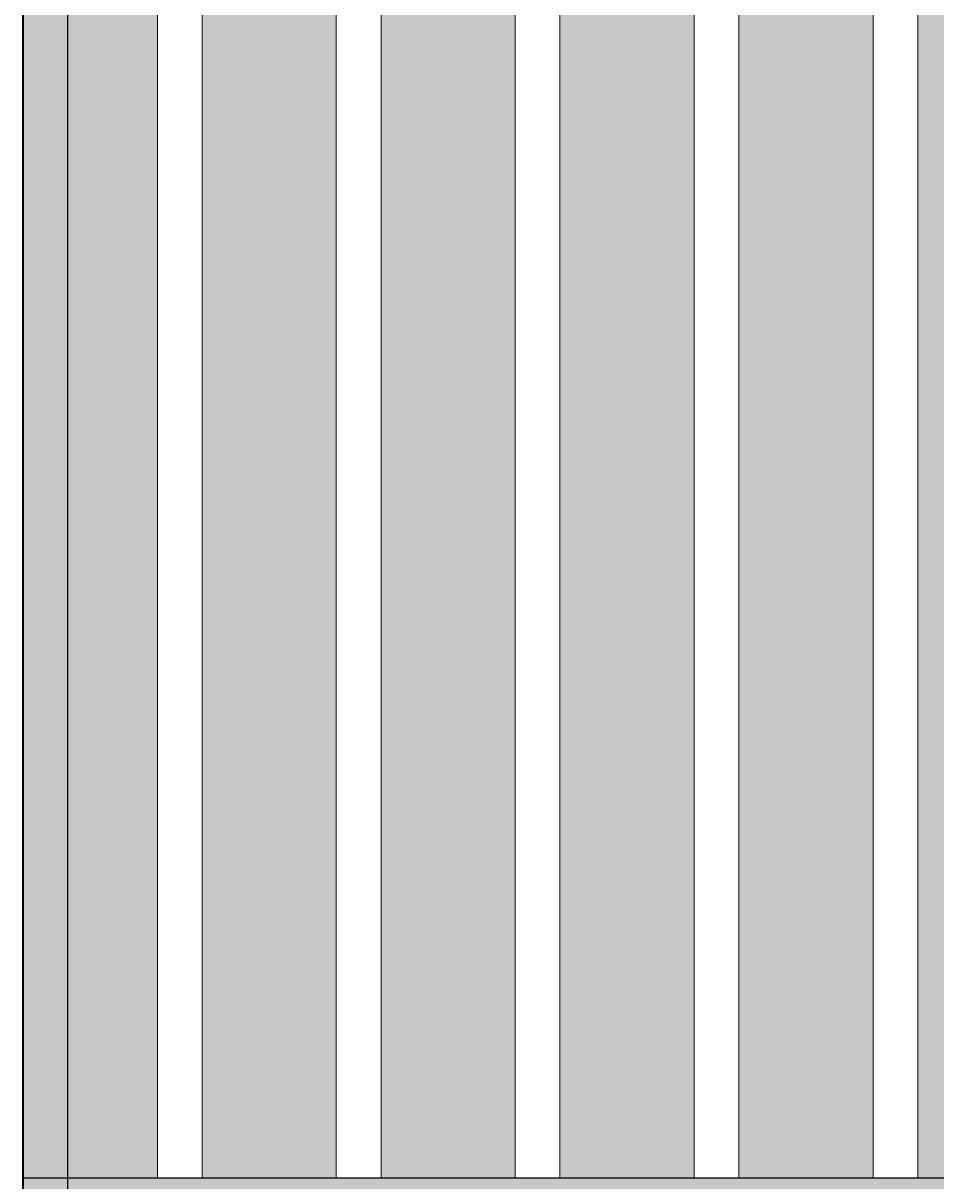
# Model space of a CAD drawing. Units: inches. Extents: x 4508 to 4723, y 847 to 1020.
# Tile 9 of 32: x 4550 to 4570, y 905 to 931. Entities that reach past the tile are written whole.
import ezdxf

# ---------------------------------------------------------------- set-up
doc = ezdxf.new("R2010")
doc.units = ezdxf.units.IN
for name, color, linetype, lineweight in [('A-ANNO-DIMS', 2, 'Continuous', 18), ('A-FURN', 8, 'Continuous', 25), ('A-WALL', 7, 'Continuous', 35), ('A-WALL-FINS', 30, 'Continuous', 18), ('A-WALL-PATT', 254, 'Continuous', 13)]:
    doc.layers.add(name, color=color, linetype=linetype, lineweight=lineweight)
doc.styles.get("Standard").update_dxf_attribs({"font": 'arial.ttf'})
doc.dimstyles.get("Standard").update_dxf_attribs({"dimtxt": 0.18, "dimasz": 0.18, "dimexe": 0.18, "dimexo": 0.0625, "dimgap": 0.09, "dimtad": 0, "dimtih": 1, "dimtoh": 1, "dimdec": 4, "dimzin": 0, "dimdsep": 46, "dimtxsty": 'Standard', "dimcen": 0.09, "dimadec": 0, "dimazin": 0, "dimtfac": 1, "dimtdec": 4, "dimtofl": 0, "dimtmove": 0, "dimatfit": 3, "dimfxl": 1, "dimtolj": 1, "dimtzin": 0, "dimarcsym": 0})

# ---------------------------------------------------------------- blocks, each defined once
blk = doc.blocks.new('*D26')
at = {"layer": 'A-ANNO-DIMS', "color": 0, "lineweight": -2, "transparency": 16777216}
for p, q in [((4549.994, 904.809), (4549.994, 1002.877)), ((4550.994, 903.809), (4550.994, 1002.877)), ((4550.174, 1002.697), (4550.371, 1002.697)), ((4550.814, 1002.697), (4550.617, 1002.697))]:
    blk.add_line(p, q, dxfattribs=at)
at = {"layer": 'A-ANNO-DIMS', "color": 0, "lineweight": 9, "transparency": 16777216}
for points in [[(4550.174, 1002.727), (4550.174, 1002.667), (4549.994, 1002.697)], [(4550.814, 1002.727), (4550.814, 1002.667), (4550.994, 1002.697)]]:
    blk.add_solid(points, dxfattribs=at)
at = {"layer": 'Defpoints', "color": 0, "lineweight": 9, "transparency": 16777216}
for p in [(4550.994, 1002.697), (4549.994, 904.747), (4550.994, 903.747)]:
    blk.add_point(p, dxfattribs=at)
at = {"layer": 'A-ANNO-DIMS', "color": 0, "transparency": 16777216, "insert": (4550.494, 1002.697), "char_height": 0.18, "attachment_point": 5}
blk.add_mtext('\\A1;1', dxfattribs=at)
blk = doc.blocks.new('*D27')
at = {"layer": 'A-ANNO-DIMS', "color": 0, "lineweight": -2, "transparency": 16777216}
for p, q in [((4550.994, 903.809), (4550.994, 1002.877)), ((4577.494, 903.809), (4577.494, 1002.877)), ((4551.174, 1002.697), (4563.918, 1002.697)), ((4577.314, 1002.697), (4564.57, 1002.697))]:
    blk.add_line(p, q, dxfattribs=at)
at = {"layer": 'A-ANNO-DIMS', "color": 0, "lineweight": 9, "transparency": 16777216}
for points in [[(4551.174, 1002.727), (4551.174, 1002.667), (4550.994, 1002.697)], [(4577.314, 1002.727), (4577.314, 1002.667), (4577.494, 1002.697)]]:
    blk.add_solid(points, dxfattribs=at)
at = {"layer": 'Defpoints', "color": 0, "lineweight": 9, "transparency": 16777216}
for p in [(4577.494, 1002.697), (4550.994, 903.747), (4577.494, 903.747)]:
    blk.add_point(p, dxfattribs=at)
at = {"layer": 'A-ANNO-DIMS', "color": 0, "transparency": 16777216, "insert": (4564.244, 1002.697), "char_height": 0.18, "attachment_point": 5}
blk.add_mtext('\\A1;26.5', dxfattribs=at)

msp = doc.modelspace()

# ---------------------------------------------------------------- hatches: boundary and pattern name
at = {"layer": 'A-WALL-PATT', "transparency": 33554681}
h = msp.add_hatch(color=256, dxfattribs=at)
h.dxf.hatch_style = 1
h.paths.add_polyline_path([(4552.9938, 994.7469), (4549.9938, 994.7469), (4549.9938, 904.7469), (4552.9938, 904.7469)])
h.paths.add_polyline_path([(4556.9938, 994.7469), (4553.9938, 994.7469), (4553.9938, 904.7469), (4556.9938, 904.7469)])
h.paths.add_polyline_path([(4560.9938, 994.7469), (4557.9938, 994.7469), (4557.9938, 904.7469), (4560.9938, 904.7469)])
h.paths.add_polyline_path([(4564.9938, 994.7469), (4561.9938, 994.7469), (4561.9938, 904.7469), (4564.9938, 904.7469)])
h.paths.add_polyline_path([(4568.9938, 994.7469), (4565.9938, 994.7469), (4565.9938, 904.7469), (4568.9938, 904.7469)])
h.paths.add_polyline_path([(4572.9938, 994.7469), (4569.9938, 994.7469), (4569.9938, 904.7469), (4572.9938, 904.7469)])
h.paths.add_polyline_path([(4576.9938, 994.7469), (4573.9938, 994.7469), (4573.9938, 904.7469), (4576.9938, 904.7469)])
h.paths.add_polyline_path([(4580.9938, 994.7469), (4577.9938, 994.7469), (4577.9938, 904.7469), (4580.9938, 904.7469)])
h.paths.add_polyline_path([(4584.9938, 994.7469), (4581.9938, 994.7469), (4581.9938, 904.7469), (4584.9938, 904.7469)])
h = msp.add_hatch(color=256, dxfattribs=at)
h.dxf.hatch_style = 1
h.paths.add_polyline_path([(4577.4938, 903.7469), (4550.9938, 903.7469), (4550.9938, 887.7469), (4577.4938, 887.7469)], flags=0)
h.paths.add_polyline_path([(4603.9938, 903.7469), (4577.9938, 903.7469), (4577.9938, 887.7469), (4603.9938, 887.7469)], flags=0)
h.paths.add_polyline_path([(4656.9938, 903.7469), (4630.9938, 903.7469), (4630.9938, 887.7469), (4656.9938, 887.7469)], flags=0)
h.paths.add_polyline_path([(4657.9938, 904.7469), (4549.9938, 904.7469), (4549.9938, 886.7469), (4657.9938, 886.7469)])
h.paths.add_polyline_path([(4656.9938, 903.7469), (4656.9938, 887.7469), (4550.9938, 887.7469), (4550.9938, 903.7469)], flags=16)

# ---------------------------------------------------------------- linework, layer by layer
at = {"layer": 'A-FURN'}
msp.add_lwpolyline([(4657.9938, 886.7469), (4549.9938, 886.7469), (4549.9938, 904.7469), (4657.9938, 904.7469)], close=True, dxfattribs=at)
at = {"layer": 'A-WALL'}
msp.add_line((4549.9938, 874.7469), (4549.9938, 994.7469), dxfattribs=at)
at = {"layer": 'A-WALL-FINS'}
for p, q in [((4552.9938, 904.7469), (4552.9938, 994.7469)), ((4553.9938, 904.7469), (4553.9938, 994.7469)), ((4556.9938, 904.7469), (4556.9938, 994.7469)), ((4557.9938, 904.7469), (4557.9938, 994.7469)), ((4560.9938, 904.7469), (4560.9938, 994.7469)), ((4561.9938, 904.7469), (4561.9938, 994.7469)), ((4564.9938, 904.7469), (4564.9938, 994.7469)), ((4565.9938, 904.7469), (4565.9938, 994.7469)), ((4568.9938, 904.7469), (4568.9938, 994.7469)), ((4569.9938, 904.7469), (4569.9938, 994.7469))]:
    msp.add_line(p, q, dxfattribs=at)

# ---------------------------------------------------------------- dimensions: what is measured, and where the dimension line sits
at = {"layer": 'A-ANNO-DIMS'}
for base, p1, p2, override, picture, middle in [((4550.9938, 1002.6969), (4549.9938, 904.7469), (4550.9938, 903.7469), {"dimdec": 0, "dimlfac": 1, "dimrnd": 0, "dimzin": 0, "dimdsep": 46, "dimlunit": 2}, '*D26', (4550.4938, 1002.6969)), ((4577.4938, 1002.6969), (4550.9938, 903.7469), (4577.4938, 903.7469), {"dimdec": 1, "dimlfac": 1, "dimrnd": 0, "dimzin": 0, "dimdsep": 46, "dimlunit": 2}, '*D27', (4564.2438, 1002.6969))]:
    dim = msp.add_linear_dim(base=base, p1=p1, p2=p2, dimstyle='Standard', override=override, dxfattribs=at)
    dim.commit()
    dim.dimension.update_dxf_attribs({"geometry": picture, "text_midpoint": middle})

doc.saveas('drawing.dxf')
